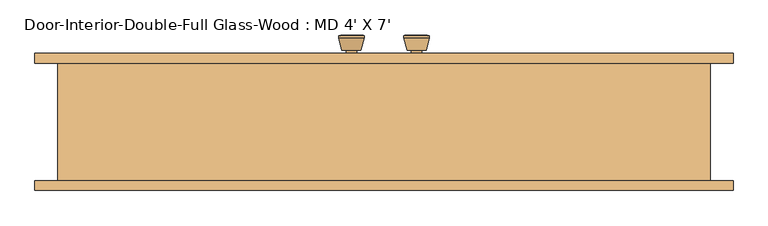
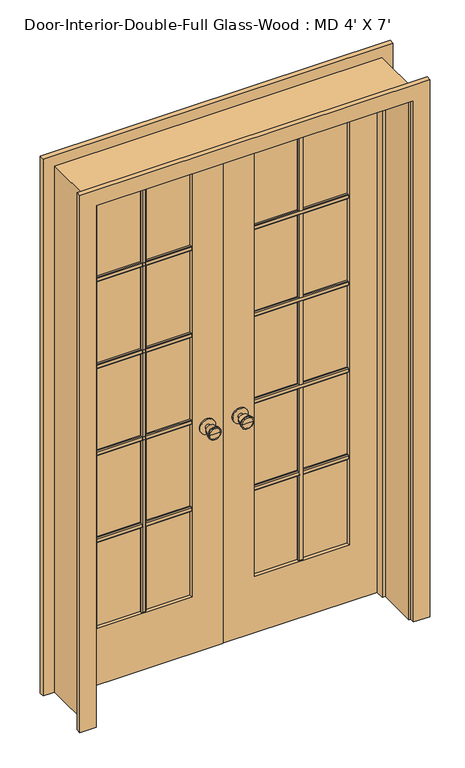
"""IFC4 building model written with IfcOpenShell, lengths in millimetres: door geometry, Door-Interior-Double-Full Glass-Wood : MD 4' X 7'."""

from ifc_helpers import new_model, si_unit, point, frame, frame_2d, origin, place, context, project, spatial, polyline, circle_curve, trimmed, segment, composite_curve, outline, extrude, faceted_brep, source, transform, mapped, element, save
from ifc_brep_helpers import plane_surface, cylinder_surface, revolved_surface, advanced_brep


def door_interior_double_full_glass_wood_md_4_x_7_6b6f14de(model_context):
    return source(origin(), model_context, "Body", "SolidModel", [
        advanced_brep(
        [(-63.5, 117.125, 914.4), (-73.5, 117.125, 914.4), (-53.5, 117.125, 914.4), (-83.9758676, 166.125, 914.4), (-63.5, 166.125, 914.4), (-43.0241324, 166.125, 914.4), (-88.5, 164.2971319, 914.4), (-38.5, 164.2971319, 914.4), (-88.5, 160.8334537, 914.4), (-38.5, 160.8334537, 914.4), (-82.136236, 136.125, 914.4), (-44.863764, 136.125, 914.4), (-73.5, 136.125, 914.4), (-53.5, 136.125, 914.4)],
        [
            (0, 1),
            (1, 2, circle_curve(frame((-63.5, 117.125, 914.4), z_axis=(0.0, -1.0, 0.0), x_axis=(1.0, 0.0, 0.0)), 10.0)),
            (2, 0),
            (2, 1, circle_curve(frame((-63.5, 117.125, 914.4), z_axis=(0.0, -1.0, 0.0), x_axis=(1.0, 0.0, 0.0)), 10.0)),
            (3, 4),
            (4, 5),
            (5, 3, circle_curve(frame((-63.5, 166.125, 914.4), z_axis=(0.0, 1.0, 0.0), x_axis=(1.0, 0.0, 0.0)), 20.4758676)),
            (3, 5, circle_curve(frame((-63.5, 166.125, 914.4), z_axis=(0.0, 1.0, 0.0), x_axis=(1.0, 0.0, 0.0)), 20.4758676)),
            (6, 3),
            (5, 7),
            (7, 6, circle_curve(frame((-63.5, 164.2971319, 914.4), z_axis=(0.0, 1.0, 0.0), x_axis=(1.0, 0.0, 0.0)), 25.0)),
            (6, 7, circle_curve(frame((-63.5, 164.2971319, 914.4), z_axis=(0.0, 1.0, 0.0), x_axis=(1.0, 0.0, 0.0)), 25.0)),
            (8, 6),
            (7, 9),
            (9, 8, circle_curve(frame((-63.5, 160.8334537, 914.4), z_axis=(0.0, 1.0, 0.0), x_axis=(1.0, 0.0, 0.0)), 25.0)),
            (8, 9, circle_curve(frame((-63.5, 160.8334537, 914.4), z_axis=(0.0, 1.0, 0.0), x_axis=(1.0, 0.0, 0.0)), 25.0)),
            (10, 8),
            (9, 11),
            (11, 10, circle_curve(frame((-63.5, 136.125, 914.4), z_axis=(0.0, 1.0, 0.0), x_axis=(1.0, 0.0, 0.0)), 18.636236)),
            (10, 11, circle_curve(frame((-63.5, 136.125, 914.4), z_axis=(0.0, 1.0, 0.0), x_axis=(1.0, 0.0, 0.0)), 18.636236)),
            (12, 10),
            (11, 13),
            (13, 12, circle_curve(frame((-63.5, 136.125, 914.4), z_axis=(0.0, 1.0, 0.0), x_axis=(1.0, 0.0, 0.0)), 10.0)),
            (12, 13, circle_curve(frame((-63.5, 136.125, 914.4), z_axis=(0.0, 1.0, 0.0), x_axis=(1.0, 0.0, 0.0)), 10.0)),
            (1, 12),
            (13, 2),
        ],
        [
            plane_surface(frame((-63.5, 117.125, 914.4), z_axis=(0.0, -1.0, 0.0), x_axis=(1.0, 0.0, 0.0))),
            plane_surface(frame((-63.5, 166.125, 914.4), z_axis=(0.0, 1.0, 0.0), x_axis=(1.0, 0.0, 0.0))),
            revolved_surface(polyline([(-43.0241324, 166.125, 914.4), (-38.5, 164.2971319, 914.4)]), (-63.5, 117.125, 914.4), (0.0, -1.0, 0.0)),
            cylinder_surface(frame((-63.5, 117.125, 914.4), z_axis=(0.0, -1.0, 0.0), x_axis=(1.0, 0.0, 0.0)), 25.0),
            revolved_surface(polyline([(-38.5, 160.8334537, 914.4), (-44.863764, 136.125, 914.4)]), (-63.5, 117.125, 914.4), (0.0, -1.0, 0.0)),
            plane_surface(frame((-63.5, 136.125, 914.4), z_axis=(0.0, -1.0, 0.0), x_axis=(1.0, 0.0, 0.0))),
            cylinder_surface(frame((-63.5, 117.125, 914.4), z_axis=(0.0, -1.0, 0.0), x_axis=(1.0, 0.0, 0.0)), 10.0),
        ],
        [
            (0, [[1, 2, 3]]),
            (0, [[-3, 4, -1]]),
            (1, [[5, 6, 7]]),
            (1, [[-6, -5, 8]]),
            (2, [[9, -7, 10, 11]]),
            (2, [[-10, -8, -9, 12]]),
            (3, [[13, -11, 14, 15]]),
            (3, [[-14, -12, -13, 16]]),
            (4, [[17, -15, 18, 19]]),
            (4, [[-18, -16, -17, 20]]),
            (5, [[21, -19, 22, 23]]),
            (5, [[-22, -20, -21, 24]]),
            (6, [[25, -23, 26, -2]]),
            (6, [[-26, -24, -25, -4]]),
        ],
    ),
        extrude(outline(composite_curve([segment(trimmed(circle_curve(frame_2d((914.4, -63.5)), 30.0), [point((914.4, -33.5))], [point((914.4, -93.5))], False, "CARTESIAN"), True, "CONTINUOUS"), segment(trimmed(circle_curve(frame_2d((914.4, -63.5)), 30.0), [point((914.4, -93.5))], [point((914.4, -33.5))], False, "CARTESIAN"), True, "CONTINUOUS")], self_intersect=False)), frame((0.0, 111.125, 0.0), z_axis=(0.0, 1.0, 0.0), x_axis=(0.0, 0.0, 1.0)), (0.0, 0.0, 1.0), 6.0),
        advanced_brep(
        [(-63.5, 70.2, 914.4), (-53.5, 70.2, 914.4), (-73.5, 70.2, 914.4), (-83.9758676, 21.2, 914.4), (-43.0241324, 21.2, 914.4), (-63.5, 21.2, 914.4), (-88.5, 23.0278681, 914.4), (-38.5, 23.0278681, 914.4), (-88.5, 26.4915463, 914.4), (-38.5, 26.4915463, 914.4), (-82.136236, 51.2, 914.4), (-44.863764, 51.2, 914.4), (-73.5, 51.2, 914.4), (-53.5, 51.2, 914.4)],
        [
            (0, 1),
            (1, 2, circle_curve(frame((-63.5, 70.2, 914.4), z_axis=(0.0, 1.0, 0.0), x_axis=(1.0, 0.0, 0.0)), 10.0)),
            (2, 0),
            (2, 1, circle_curve(frame((-63.5, 70.2, 914.4), z_axis=(0.0, 1.0, 0.0), x_axis=(1.0, 0.0, 0.0)), 10.0)),
            (3, 4, circle_curve(frame((-63.5, 21.2, 914.4), z_axis=(0.0, -1.0, 0.0), x_axis=(1.0, 0.0, 0.0)), 20.4758676)),
            (4, 5),
            (5, 3),
            (4, 3, circle_curve(frame((-63.5, 21.2, 914.4), z_axis=(0.0, -1.0, 0.0), x_axis=(1.0, 0.0, 0.0)), 20.4758676)),
            (6, 7, circle_curve(frame((-63.5, 23.0278681, 914.4), z_axis=(0.0, -1.0, 0.0), x_axis=(1.0, 0.0, 0.0)), 25.0)),
            (7, 4),
            (3, 6),
            (7, 6, circle_curve(frame((-63.5, 23.0278681, 914.4), z_axis=(0.0, -1.0, 0.0), x_axis=(1.0, 0.0, 0.0)), 25.0)),
            (8, 9, circle_curve(frame((-63.5, 26.4915463, 914.4), z_axis=(0.0, -1.0, 0.0), x_axis=(1.0, 0.0, 0.0)), 25.0)),
            (9, 7),
            (6, 8),
            (9, 8, circle_curve(frame((-63.5, 26.4915463, 914.4), z_axis=(0.0, -1.0, 0.0), x_axis=(1.0, 0.0, 0.0)), 25.0)),
            (10, 11, circle_curve(frame((-63.5, 51.2, 914.4), z_axis=(0.0, -1.0, 0.0), x_axis=(1.0, 0.0, 0.0)), 18.636236)),
            (11, 9),
            (8, 10),
            (11, 10, circle_curve(frame((-63.5, 51.2, 914.4), z_axis=(0.0, -1.0, 0.0), x_axis=(1.0, 0.0, 0.0)), 18.636236)),
            (12, 13, circle_curve(frame((-63.5, 51.2, 914.4), z_axis=(0.0, -1.0, 0.0), x_axis=(1.0, 0.0, 0.0)), 10.0)),
            (13, 11),
            (10, 12),
            (13, 12, circle_curve(frame((-63.5, 51.2, 914.4), z_axis=(0.0, -1.0, 0.0), x_axis=(1.0, 0.0, 0.0)), 10.0)),
            (1, 13),
            (12, 2),
        ],
        [
            plane_surface(frame((-63.5, 70.2, 914.4), z_axis=(0.0, 1.0, 0.0), x_axis=(1.0, 0.0, 0.0))),
            plane_surface(frame((-63.5, 21.2, 914.4), z_axis=(0.0, -1.0, 0.0), x_axis=(1.0, 0.0, 0.0))),
            revolved_surface(polyline([(-43.0241324, 21.2, 914.4), (-38.5, 23.0278681, 914.4)]), (-63.5, 70.2, 914.4), (0.0, 1.0, 0.0)),
            cylinder_surface(frame((-63.5, 70.2, 914.4), z_axis=(0.0, 1.0, 0.0), x_axis=(1.0, 0.0, 0.0)), 25.0),
            revolved_surface(polyline([(-38.5, 26.4915463, 914.4), (-44.863764, 51.2, 914.4)]), (-63.5, 70.2, 914.4), (0.0, 1.0, 0.0)),
            plane_surface(frame((-63.5, 51.2, 914.4), z_axis=(0.0, 1.0, 0.0), x_axis=(1.0, 0.0, 0.0))),
            cylinder_surface(frame((-63.5, 70.2, 914.4), z_axis=(0.0, 1.0, 0.0), x_axis=(1.0, 0.0, 0.0)), 10.0),
        ],
        [
            (0, [[1, 2, 3]]),
            (0, [[-3, 4, -1]]),
            (1, [[5, 6, 7]]),
            (1, [[8, -7, -6]]),
            (2, [[9, 10, -5, 11]]),
            (2, [[12, -11, -8, -10]]),
            (3, [[13, 14, -9, 15]]),
            (3, [[16, -15, -12, -14]]),
            (4, [[17, 18, -13, 19]]),
            (4, [[20, -19, -16, -18]]),
            (5, [[21, 22, -17, 23]]),
            (5, [[24, -23, -20, -22]]),
            (6, [[-2, 25, -21, 26]]),
            (6, [[-4, -26, -24, -25]]),
        ],
    ),
        extrude(outline(composite_curve([segment(trimmed(circle_curve(frame_2d((914.4, -63.5)), 30.0), [point((914.4, -33.5))], [point((914.4, -93.5))], False, "CARTESIAN"), True, "CONTINUOUS"), segment(trimmed(circle_curve(frame_2d((914.4, -63.5)), 30.0), [point((914.4, -93.5))], [point((914.4, -33.5))], False, "CARTESIAN"), True, "CONTINUOUS")], self_intersect=False)), frame((0.0, 70.2, 0.0), z_axis=(0.0, 1.0, 0.0), x_axis=(0.0, 0.0, 1.0)), (0.0, 0.0, 1.0), 6.0),
        extrude(outline(polyline([(90.17, 1667.51), (90.17, 1648.46), (83.82, 1648.46), (80.645, 1651.635), (80.645, 1664.335), (83.82, 1667.51), (90.17, 1667.51)])), frame((120.65, 0.0, 0.0), z_axis=(1.0, 0.0, 0.0), x_axis=(0.0, 1.0, 0.0)), (0.0, 0.0, 1.0), 368.3),
        extrude(outline(polyline([(90.17, 1310.9575), (90.17, 1291.9075), (83.82, 1291.9075), (80.645, 1295.0825), (80.645, 1307.7825), (83.82, 1310.9575), (90.17, 1310.9575)])), frame((120.65, 0.0, 0.0), z_axis=(1.0, 0.0, 0.0), x_axis=(0.0, 1.0, 0.0)), (0.0, 0.0, 1.0), 368.3),
        extrude(outline(polyline([(90.17, 954.405), (90.17, 935.355), (83.82, 935.355), (80.645, 938.53), (80.645, 951.23), (83.82, 954.405), (90.17, 954.405)])), frame((120.65, 0.0, 0.0), z_axis=(1.0, 0.0, 0.0), x_axis=(0.0, 1.0, 0.0)), (0.0, 0.0, 1.0), 368.3),
        extrude(outline(polyline([(295.275, 90.17), (314.325, 90.17), (314.325, 83.82), (311.15, 80.645), (298.45, 80.645), (295.275, 83.82), (295.275, 90.17)])), frame((0.0, 0.0, 231.775), z_axis=(0.0, 0.0, 1.0), x_axis=(1.0, 0.0, 0.0)), (0.0, 0.0, 1.0), 1782.7625),
        extrude(outline(polyline([(90.17, 597.8525), (90.17, 578.8025), (83.82, 578.8025), (80.645, 581.9775), (80.645, 594.6775), (83.82, 597.8525), (90.17, 597.8525)])), frame((120.65, 0.0, 0.0), z_axis=(1.0, 0.0, 0.0), x_axis=(0.0, 1.0, 0.0)), (0.0, 0.0, 1.0), 368.3),
        extrude(outline(polyline([(97.155, 1667.51), (103.505, 1667.51), (106.68, 1664.335), (106.68, 1651.635), (103.505, 1648.46), (97.155, 1648.46), (97.155, 1667.51)])), frame((-488.95, 0.0, 0.0), z_axis=(1.0, 0.0, 0.0), x_axis=(0.0, 1.0, 0.0)), (0.0, 0.0, 1.0), 368.3),
        extrude(outline(polyline([(97.155, 1310.9575), (103.505, 1310.9575), (106.68, 1307.7825), (106.68, 1295.0825), (103.505, 1291.9075), (97.155, 1291.9075), (97.155, 1310.9575)])), frame((-488.95, 0.0, 0.0), z_axis=(1.0, 0.0, 0.0), x_axis=(0.0, 1.0, 0.0)), (0.0, 0.0, 1.0), 368.3),
        extrude(outline(polyline([(97.155, 954.405), (103.505, 954.405), (106.68, 951.23), (106.68, 938.53), (103.505, 935.355), (97.155, 935.355), (97.155, 954.405)])), frame((-488.95, 0.0, 0.0), z_axis=(1.0, 0.0, 0.0), x_axis=(0.0, 1.0, 0.0)), (0.0, 0.0, 1.0), 368.3),
        extrude(outline(polyline([(-314.325, 97.155), (-314.325, 103.505), (-311.15, 106.68), (-298.45, 106.68), (-295.275, 103.505), (-295.275, 97.155), (-314.325, 97.155)])), frame((0.0, 0.0, 231.775), z_axis=(0.0, 0.0, 1.0), x_axis=(1.0, 0.0, 0.0)), (0.0, 0.0, 1.0), 1782.7625),
        extrude(outline(polyline([(97.155, 597.8525), (103.505, 597.8525), (106.68, 594.6775), (106.68, 581.9775), (103.505, 578.8025), (97.155, 578.8025), (97.155, 597.8525)])), frame((-488.95, 0.0, 0.0), z_axis=(1.0, 0.0, 0.0), x_axis=(0.0, 1.0, 0.0)), (0.0, 0.0, 1.0), 368.3),
        extrude(outline(polyline([(97.155, 1667.51), (103.505, 1667.51), (106.68, 1664.335), (106.68, 1651.635), (103.505, 1648.46), (97.155, 1648.46), (97.155, 1667.51)])), frame((120.65, 0.0, 0.0), z_axis=(1.0, 0.0, 0.0), x_axis=(0.0, 1.0, 0.0)), (0.0, 0.0, 1.0), 368.3),
        extrude(outline(polyline([(97.155, 1310.9575), (103.505, 1310.9575), (106.68, 1307.7825), (106.68, 1295.0825), (103.505, 1291.9075), (97.155, 1291.9075), (97.155, 1310.9575)])), frame((120.65, 0.0, 0.0), z_axis=(1.0, 0.0, 0.0), x_axis=(0.0, 1.0, 0.0)), (0.0, 0.0, 1.0), 368.3),
        extrude(outline(polyline([(97.155, 954.405), (103.505, 954.405), (106.68, 951.23), (106.68, 938.53), (103.505, 935.355), (97.155, 935.355), (97.155, 954.405)])), frame((120.65, 0.0, 0.0), z_axis=(1.0, 0.0, 0.0), x_axis=(0.0, 1.0, 0.0)), (0.0, 0.0, 1.0), 368.3),
        extrude(outline(polyline([(295.275, 97.155), (295.275, 103.505), (298.45, 106.68), (311.15, 106.68), (314.325, 103.505), (314.325, 97.155), (295.275, 97.155)])), frame((0.0, 0.0, 231.775), z_axis=(0.0, 0.0, 1.0), x_axis=(1.0, 0.0, 0.0)), (0.0, 0.0, 1.0), 1782.7625),
        extrude(outline(polyline([(97.155, 597.8525), (103.505, 597.8525), (106.68, 594.6775), (106.68, 581.9775), (103.505, 578.8025), (97.155, 578.8025), (97.155, 597.8525)])), frame((120.65, 0.0, 0.0), z_axis=(1.0, 0.0, 0.0), x_axis=(0.0, 1.0, 0.0)), (0.0, 0.0, 1.0), 368.3),
        extrude(outline(polyline([(90.17, 1667.51), (90.17, 1648.46), (83.82, 1648.46), (80.645, 1651.635), (80.645, 1664.335), (83.82, 1667.51), (90.17, 1667.51)])), frame((-488.95, 0.0, 0.0), z_axis=(1.0, 0.0, 0.0), x_axis=(0.0, 1.0, 0.0)), (0.0, 0.0, 1.0), 368.3),
        extrude(outline(polyline([(90.17, 1310.9575), (90.17, 1291.9075), (83.82, 1291.9075), (80.645, 1295.0825), (80.645, 1307.7825), (83.82, 1310.9575), (90.17, 1310.9575)])), frame((-488.95, 0.0, 0.0), z_axis=(1.0, 0.0, 0.0), x_axis=(0.0, 1.0, 0.0)), (0.0, 0.0, 1.0), 368.3),
        extrude(outline(polyline([(90.17, 954.405), (90.17, 935.355), (83.82, 935.355), (80.645, 938.53), (80.645, 951.23), (83.82, 954.405), (90.17, 954.405)])), frame((-488.95, 0.0, 0.0), z_axis=(1.0, 0.0, 0.0), x_axis=(0.0, 1.0, 0.0)), (0.0, 0.0, 1.0), 368.3),
        extrude(outline(polyline([(-314.325, 90.17), (-295.275, 90.17), (-295.275, 83.82), (-298.45, 80.645), (-311.15, 80.645), (-314.325, 83.82), (-314.325, 90.17)])), frame((0.0, 0.0, 231.775), z_axis=(0.0, 0.0, 1.0), x_axis=(1.0, 0.0, 0.0)), (0.0, 0.0, 1.0), 1782.7625),
        extrude(outline(polyline([(90.17, 597.8525), (90.17, 578.8025), (83.82, 578.8025), (80.645, 581.9775), (80.645, 594.6775), (83.82, 597.8525), (90.17, 597.8525)])), frame((-488.95, 0.0, 0.0), z_axis=(1.0, 0.0, 0.0), x_axis=(0.0, 1.0, 0.0)), (0.0, 0.0, 1.0), 368.3),
        advanced_brep(
        [(63.5, 70.2, 914.4), (73.5, 70.2, 914.4), (53.5, 70.2, 914.4), (83.9758676, 21.2, 914.4), (63.5, 21.2, 914.4), (43.0241324, 21.2, 914.4), (88.5, 23.0278681, 914.4), (38.5, 23.0278681, 914.4), (88.5, 26.4915463, 914.4), (38.5, 26.4915463, 914.4), (82.136236, 51.2, 914.4), (44.863764, 51.2, 914.4), (73.5, 51.2, 914.4), (53.5, 51.2, 914.4)],
        [
            (0, 1),
            (1, 2, circle_curve(frame((63.5, 70.2, 914.4), z_axis=(0.0, 1.0, 0.0), x_axis=(-1.0, 0.0, 0.0)), 10.0)),
            (2, 0),
            (2, 1, circle_curve(frame((63.5, 70.2, 914.4), z_axis=(0.0, 1.0, 0.0), x_axis=(-1.0, 0.0, 0.0)), 10.0)),
            (3, 4),
            (4, 5),
            (5, 3, circle_curve(frame((63.5, 21.2, 914.4), z_axis=(0.0, -1.0, 0.0), x_axis=(-1.0, 0.0, 0.0)), 20.4758676)),
            (3, 5, circle_curve(frame((63.5, 21.2, 914.4), z_axis=(0.0, -1.0, 0.0), x_axis=(-1.0, 0.0, 0.0)), 20.4758676)),
            (6, 3),
            (5, 7),
            (7, 6, circle_curve(frame((63.5, 23.0278681, 914.4), z_axis=(0.0, -1.0, 0.0), x_axis=(-1.0, 0.0, 0.0)), 25.0)),
            (6, 7, circle_curve(frame((63.5, 23.0278681, 914.4), z_axis=(0.0, -1.0, 0.0), x_axis=(-1.0, 0.0, 0.0)), 25.0)),
            (8, 6),
            (7, 9),
            (9, 8, circle_curve(frame((63.5, 26.4915463, 914.4), z_axis=(0.0, -1.0, 0.0), x_axis=(-1.0, 0.0, 0.0)), 25.0)),
            (8, 9, circle_curve(frame((63.5, 26.4915463, 914.4), z_axis=(0.0, -1.0, 0.0), x_axis=(-1.0, 0.0, 0.0)), 25.0)),
            (10, 8),
            (9, 11),
            (11, 10, circle_curve(frame((63.5, 51.2, 914.4), z_axis=(0.0, -1.0, 0.0), x_axis=(-1.0, 0.0, 0.0)), 18.636236)),
            (10, 11, circle_curve(frame((63.5, 51.2, 914.4), z_axis=(0.0, -1.0, 0.0), x_axis=(-1.0, 0.0, 0.0)), 18.636236)),
            (12, 10),
            (11, 13),
            (13, 12, circle_curve(frame((63.5, 51.2, 914.4), z_axis=(0.0, -1.0, 0.0), x_axis=(-1.0, 0.0, 0.0)), 10.0)),
            (12, 13, circle_curve(frame((63.5, 51.2, 914.4), z_axis=(0.0, -1.0, 0.0), x_axis=(-1.0, 0.0, 0.0)), 10.0)),
            (1, 12),
            (13, 2),
        ],
        [
            plane_surface(frame((63.5, 70.2, 914.4), z_axis=(0.0, 1.0, 0.0), x_axis=(-1.0, 0.0, 0.0))),
            plane_surface(frame((63.5, 21.2, 914.4), z_axis=(0.0, -1.0, 0.0), x_axis=(-1.0, 0.0, 0.0))),
            revolved_surface(polyline([(43.0241324, 21.2, 914.4), (38.5, 23.0278681, 914.4)]), (63.5, 70.2, 914.4), (0.0, 1.0, 0.0)),
            cylinder_surface(frame((63.5, 70.2, 914.4), z_axis=(0.0, 1.0, 0.0), x_axis=(-1.0, 0.0, 0.0)), 25.0),
            revolved_surface(polyline([(38.5, 26.4915463, 914.4), (44.863764, 51.2, 914.4)]), (63.5, 70.2, 914.4), (0.0, 1.0, 0.0)),
            plane_surface(frame((63.5, 51.2, 914.4), z_axis=(0.0, 1.0, 0.0), x_axis=(-1.0, 0.0, 0.0))),
            cylinder_surface(frame((63.5, 70.2, 914.4), z_axis=(0.0, 1.0, 0.0), x_axis=(-1.0, 0.0, 0.0)), 10.0),
        ],
        [
            (0, [[1, 2, 3]]),
            (0, [[-3, 4, -1]]),
            (1, [[5, 6, 7]]),
            (1, [[-6, -5, 8]]),
            (2, [[9, -7, 10, 11]]),
            (2, [[-10, -8, -9, 12]]),
            (3, [[13, -11, 14, 15]]),
            (3, [[-14, -12, -13, 16]]),
            (4, [[17, -15, 18, 19]]),
            (4, [[-18, -16, -17, 20]]),
            (5, [[21, -19, 22, 23]]),
            (5, [[-22, -20, -21, 24]]),
            (6, [[25, -23, 26, -2]]),
            (6, [[-26, -24, -25, -4]]),
        ],
    ),
        extrude(outline(composite_curve([segment(trimmed(circle_curve(frame_2d((914.4, 63.5)), 30.0), [point((914.4, 33.5))], [point((914.4, 93.5))], False, "CARTESIAN"), True, "CONTINUOUS"), segment(trimmed(circle_curve(frame_2d((914.4, 63.5)), 30.0), [point((914.4, 93.5))], [point((914.4, 33.5))], False, "CARTESIAN"), True, "CONTINUOUS")], self_intersect=False)), frame((0.0, 70.2, 0.0), z_axis=(0.0, 1.0, 0.0), x_axis=(0.0, 0.0, 1.0)), (0.0, 0.0, 1.0), 6.0),
        advanced_brep(
        [(63.5, 117.125, 914.4), (53.5, 117.125, 914.4), (73.5, 117.125, 914.4), (83.9758676, 166.125, 914.4), (43.0241324, 166.125, 914.4), (63.5, 166.125, 914.4), (88.5, 164.2971319, 914.4), (38.5, 164.2971319, 914.4), (88.5, 160.8334537, 914.4), (38.5, 160.8334537, 914.4), (82.136236, 136.125, 914.4), (44.863764, 136.125, 914.4), (73.5, 136.125, 914.4), (53.5, 136.125, 914.4)],
        [
            (0, 1),
            (1, 2, circle_curve(frame((63.5, 117.125, 914.4), z_axis=(0.0, -1.0, 0.0), x_axis=(-1.0, 0.0, 0.0)), 10.0)),
            (2, 0),
            (2, 1, circle_curve(frame((63.5, 117.125, 914.4), z_axis=(0.0, -1.0, 0.0), x_axis=(-1.0, 0.0, 0.0)), 10.0)),
            (3, 4, circle_curve(frame((63.5, 166.125, 914.4), z_axis=(0.0, 1.0, 0.0), x_axis=(-1.0, 0.0, 0.0)), 20.4758676)),
            (4, 5),
            (5, 3),
            (4, 3, circle_curve(frame((63.5, 166.125, 914.4), z_axis=(0.0, 1.0, 0.0), x_axis=(-1.0, 0.0, 0.0)), 20.4758676)),
            (6, 7, circle_curve(frame((63.5, 164.2971319, 914.4), z_axis=(0.0, 1.0, 0.0), x_axis=(-1.0, 0.0, 0.0)), 25.0)),
            (7, 4),
            (3, 6),
            (7, 6, circle_curve(frame((63.5, 164.2971319, 914.4), z_axis=(0.0, 1.0, 0.0), x_axis=(-1.0, 0.0, 0.0)), 25.0)),
            (8, 9, circle_curve(frame((63.5, 160.8334537, 914.4), z_axis=(0.0, 1.0, 0.0), x_axis=(-1.0, 0.0, 0.0)), 25.0)),
            (9, 7),
            (6, 8),
            (9, 8, circle_curve(frame((63.5, 160.8334537, 914.4), z_axis=(0.0, 1.0, 0.0), x_axis=(-1.0, 0.0, 0.0)), 25.0)),
            (10, 11, circle_curve(frame((63.5, 136.125, 914.4), z_axis=(0.0, 1.0, 0.0), x_axis=(-1.0, 0.0, 0.0)), 18.636236)),
            (11, 9),
            (8, 10),
            (11, 10, circle_curve(frame((63.5, 136.125, 914.4), z_axis=(0.0, 1.0, 0.0), x_axis=(-1.0, 0.0, 0.0)), 18.636236)),
            (12, 13, circle_curve(frame((63.5, 136.125, 914.4), z_axis=(0.0, 1.0, 0.0), x_axis=(-1.0, 0.0, 0.0)), 10.0)),
            (13, 11),
            (10, 12),
            (13, 12, circle_curve(frame((63.5, 136.125, 914.4), z_axis=(0.0, 1.0, 0.0), x_axis=(-1.0, 0.0, 0.0)), 10.0)),
            (1, 13),
            (12, 2),
        ],
        [
            plane_surface(frame((63.5, 117.125, 914.4), z_axis=(0.0, -1.0, 0.0), x_axis=(-1.0, 0.0, 0.0))),
            plane_surface(frame((63.5, 166.125, 914.4), z_axis=(0.0, 1.0, 0.0), x_axis=(-1.0, 0.0, 0.0))),
            revolved_surface(polyline([(43.0241324, 166.125, 914.4), (38.5, 164.2971319, 914.4)]), (63.5, 117.125, 914.4), (0.0, -1.0, 0.0)),
            cylinder_surface(frame((63.5, 117.125, 914.4), z_axis=(0.0, -1.0, 0.0), x_axis=(-1.0, 0.0, 0.0)), 25.0),
            revolved_surface(polyline([(38.5, 160.8334537, 914.4), (44.863764, 136.125, 914.4)]), (63.5, 117.125, 914.4), (0.0, -1.0, 0.0)),
            plane_surface(frame((63.5, 136.125, 914.4), z_axis=(0.0, -1.0, 0.0), x_axis=(-1.0, 0.0, 0.0))),
            cylinder_surface(frame((63.5, 117.125, 914.4), z_axis=(0.0, -1.0, 0.0), x_axis=(-1.0, 0.0, 0.0)), 10.0),
        ],
        [
            (0, [[1, 2, 3]]),
            (0, [[-3, 4, -1]]),
            (1, [[5, 6, 7]]),
            (1, [[8, -7, -6]]),
            (2, [[9, 10, -5, 11]]),
            (2, [[12, -11, -8, -10]]),
            (3, [[13, 14, -9, 15]]),
            (3, [[16, -15, -12, -14]]),
            (4, [[17, 18, -13, 19]]),
            (4, [[20, -19, -16, -18]]),
            (5, [[21, 22, -17, 23]]),
            (5, [[24, -23, -20, -22]]),
            (6, [[-2, 25, -21, 26]]),
            (6, [[-4, -26, -24, -25]]),
        ],
    ),
        extrude(outline(composite_curve([segment(trimmed(circle_curve(frame_2d((914.4, 63.5)), 30.0), [point((914.4, 33.5))], [point((914.4, 93.5))], False, "CARTESIAN"), True, "CONTINUOUS"), segment(trimmed(circle_curve(frame_2d((914.4, 63.5)), 30.0), [point((914.4, 93.5))], [point((914.4, 33.5))], False, "CARTESIAN"), True, "CONTINUOUS")], self_intersect=False)), frame((0.0, 111.125, 0.0), z_axis=(0.0, 1.0, 0.0), x_axis=(0.0, 0.0, 1.0)), (0.0, 0.0, 1.0), 6.0),
        extrude(outline(polyline([(0.0, 615.95), (0.0, 679.45), (2203.45, 679.45), (2203.45, -679.45), (0.0, -679.45), (0.0, -615.95), (2139.95, -615.95), (2139.95, 615.95), (0.0, 615.95)])), frame((0.0, -136.525, 0.0), z_axis=(0.0, 1.0, 0.0), x_axis=(0.0, 0.0, 1.0)), (0.0, 0.0, 1.0), 19.05),
        extrude(outline(polyline([(0.0, 615.95), (0.0, 679.45), (2203.45, 679.45), (2203.45, -679.45), (0.0, -679.45), (0.0, -615.95), (2139.95, -615.95), (2139.95, 615.95), (0.0, 615.95)])), frame((0.0, 111.125, 0.0), z_axis=(0.0, 1.0, 0.0), x_axis=(0.0, 0.0, 1.0)), (0.0, 0.0, 1.0), 19.05),
        faceted_brep([(635.0, 111.125, 0.0), (635.0, -117.475, 0.0), (609.6, -117.475, 0.0), (609.6, 41.275, 0.0), (596.9, 41.275, 0.0), (596.9, 76.2, 0.0), (609.6, 76.2, 0.0), (609.6, 111.125, 0.0), (635.0, 111.125, 2159.0), (635.0, -117.475, 2159.0), (-635.0, -117.475, 2159.0), (-635.0, -117.475, 0.0), (-609.6, -117.475, 0.0), (-609.6, -117.475, 2133.6), (609.6, -117.475, 2133.6), (609.6, 41.275, 2133.6), (-609.6, 41.275, 2133.6), (-609.6, 41.275, 0.0), (-596.9, 41.275, 0.0), (-596.9, 41.275, 2120.9), (596.9, 41.275, 2120.9), (596.9, 76.2, 2120.9), (1.5875, 76.2, 2120.9), (-1.6019111, 76.2, 2120.9), (-596.9, 76.2, 2120.9), (-596.9, 76.2, 0.0), (-609.6, 76.2, 0.0), (-609.6, 76.2, 2133.6), (-1.6019111, 76.2, 2133.6), (1.5875, 76.2, 2133.6), (609.6, 76.2, 2133.6), (609.6, 111.125, 2133.6), (1.5875, 111.125, 2133.6), (-1.6019111, 111.125, 2133.6), (-609.6, 111.125, 2133.6), (-609.6, 111.125, 0.0), (-635.0, 111.125, 0.0), (-635.0, 111.125, 2159.0)], [[[0, 1, 2, 3, 4, 5, 6, 7]], [[1, 0, 8, 9]], [[2, 1, 9, 10, 11, 12, 13, 14]], [[3, 2, 14, 15]], [[4, 3, 15, 16, 17, 18, 19, 20]], [[5, 4, 20, 21]], [[6, 5, 21, 22, 23, 24, 25, 26, 27, 28, 29, 30]], [[7, 6, 30, 31]], [[0, 7, 31, 32, 33, 34, 35, 36, 37, 8]], [[9, 8, 37, 10]], [[14, 13, 16, 15]], [[20, 19, 24, 23, 22, 21]], [[31, 30, 29, 28, 27, 34, 33, 32]], [[12, 11, 36, 35, 26, 25, 18, 17]], [[11, 10, 37, 36]], [[13, 12, 17, 16]], [[19, 18, 25, 24]], [[27, 26, 35, 34]]]),
        extrude(outline(polyline([(2133.6, -609.6), (0.0, -609.6), (0.0, -1.6019111), (2133.6, -1.6019111), (2133.6, -609.6)]), holes=[polyline([(231.775, -488.95), (2014.5375, -488.95), (2014.5375, -120.65), (231.775, -120.65), (231.775, -488.95)])]), frame((0.0, 76.2, 0.0), z_axis=(0.0, 1.0, 0.0), x_axis=(0.0, 0.0, 1.0)), (0.0, 0.0, 1.0), 34.925),
        extrude(outline(polyline([(0.0, 609.6), (2133.6, 609.6), (2133.6, 1.5875), (0.0, 1.5875), (0.0, 609.6)]), holes=[polyline([(2014.5375, 120.65), (2014.5375, 488.95), (231.775, 488.95), (231.775, 120.65), (2014.5375, 120.65)])]), frame((0.0, 76.2, 0.0), z_axis=(0.0, 1.0, 0.0), x_axis=(0.0, 0.0, 1.0)), (0.0, 0.0, 1.0), 34.925),
        extrude(outline(polyline([(488.95, 90.17), (120.65, 90.17), (120.65, 97.155), (488.95, 97.155), (488.95, 90.17)])), frame((0.0, 0.0, 231.775), z_axis=(0.0, 0.0, 1.0), x_axis=(1.0, 0.0, 0.0)), (0.0, 0.0, 1.0), 1782.7625),
        extrude(outline(polyline([(-120.65, 90.17), (-488.95, 90.17), (-488.95, 97.155), (-120.65, 97.155), (-120.65, 90.17)])), frame((0.0, 0.0, 231.775), z_axis=(0.0, 0.0, 1.0), x_axis=(1.0, 0.0, 0.0)), (0.0, 0.0, 1.0), 1782.7625),
    ])


if __name__ == "__main__":
    model = new_model("IFC4")
    model_context = context("Model", 3, world=origin())
    ifc_project = project(units=[si_unit("LENGTHUNIT", "METRE", prefix="MILLI")], contexts=[model_context])
    site = spatial("IfcSite", under=ifc_project)
    building = spatial("IfcBuilding", under=site)
    placement = place(None, origin())
    door_interior_double_full_glass_wood_md_4_x_7_shape = door_interior_double_full_glass_wood_md_4_x_7_6b6f14de(model_context)
    element("IfcDoor", 1, ObjectType="Door-Interior-Double-Full Glass-Wood : MD 4' X 7'", at=placement, inside=building, context=model_context, shape_type="MappedRepresentation", body=[
        mapped(door_interior_double_full_glass_wood_md_4_x_7_shape, transform((0.0, 0.0, 0.0), x_axis=(1.0, 0.0, 0.0), y_axis=(0.0, 1.0, 0.0), z_axis=(0.0, 0.0, 1.0))),
    ])
    save(model, "model.ifc")

# Revit data of these elements
# Type "Door-Interior-Double-Full Glass-Wood : MD 4' X 7'"
#   Type Mark = "9"
#   Assembly Code = "C1020300"
#   Analytic Construction = "French door, wood frame with single glass"
#   Top Rail = 0' - 4 11/16"
#   Thickness = 0' - 1 3/8"
#   Thermal Resistance (R) = 1.0696 (h·ft²·°F)/BTU
#   Swing Angle [instance default] = 90.00°
#   Stiles = 0' - 4 3/4"
#   Rough Width = 4' - 2"
#   Rough Height = 7' - 1"
#   Panel Width = 2' - 0"
#   Height = 7' - 0"
#   Width = 4' - 0"
#   Heat Transfer Coefficient (U) = 0.9350 BTU/(h·ft²·°F)
#   Bottom Rail = 0' - 9 1/8"
#   Show Grill [instance default] = yes
#   Trim Material = Cherry
#   Panel Material = Cherry
#   Frame Material = Cherry
#   Door Handle Material = Aluminum
#   Visual Light Transmittance = 0
#   Solar Heat Gain Coefficient = 0
#   Wall Closure = (empty or 0)
#   Function = (empty or 0)
# Element 1 (IfcDoor, "Door-Interior-Double-Full Glass-Wood : MD 4' X 7'")
#   Materials on its faces: "Cherry", "Aluminum", "Glass"
# Materials
#   "Cherry": class "Wood", colour RGB 226 177 128, transparency 0, Description = "Prunus Serotina", Cost = 0
#   "Aluminum": class "Metal", colour RGB 247 247 247, transparency 0, Description = "Aluminum 6061", Cost = 0
#   "Glass": class "Glass", colour RGB 0 128 192, transparency 0.75, Description = "Soda Lime Glass", Cost = 0
